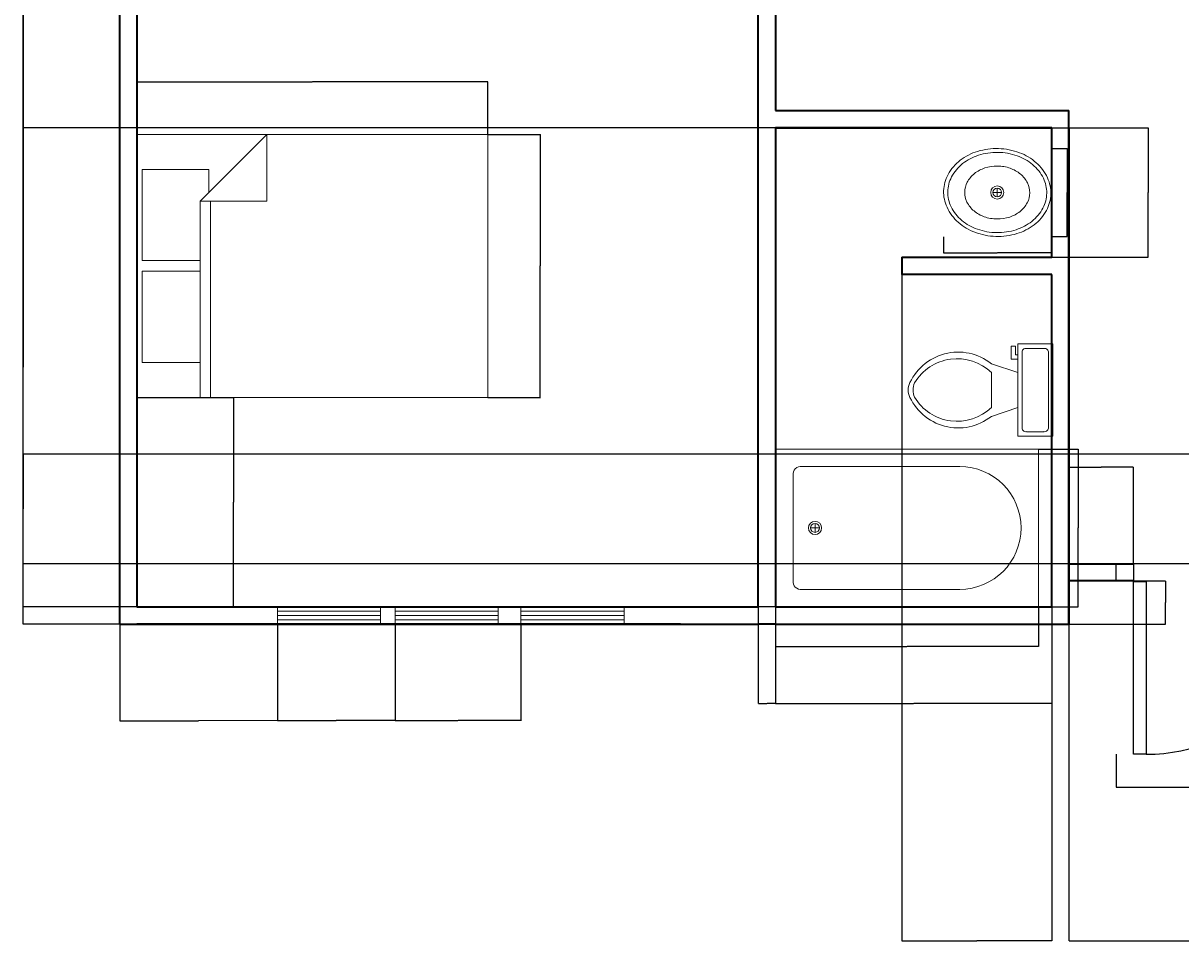
# Model space of a CAD drawing. Units: millimetres. Extents: x 1312 to 12932, y -881 to 10062.
# Tile 1 of 4: x 1312 to 8020, y -881 to 4434. Entities that reach past the tile are written whole.
import ezdxf

# ---------------------------------------------------------------- set-up
doc = ezdxf.new("R2010")
doc.units = ezdxf.units.MM
for name, color, linetype, lineweight in [('A-ANNO-DIMS', 2, 'Continuous', 18), ('A-DOOR', 3, 'Continuous', 25), ('A-FLOR-FIXT', 9, 'Continuous', 18), ('A-FURN', 8, 'Continuous', 18), ('A-GLAZ', 4, 'Continuous', 18), ('A-WALL', 7, 'Continuous', 35)]:
    doc.layers.add(name, color=color, linetype=linetype, lineweight=lineweight)
doc.styles.get("Standard").update_dxf_attribs({"font": 'arial.ttf'})
doc.dimstyles.get("Standard").update_dxf_attribs({"dimtxt": 0.18, "dimasz": 0.18, "dimexe": 0.18, "dimexo": 0.0625, "dimgap": 0.09, "dimtad": 0, "dimtih": 1, "dimtoh": 1, "dimdec": 4, "dimzin": 0, "dimdsep": 46, "dimtxsty": 'Standard', "dimcen": 0.09, "dimadec": 0, "dimazin": 0, "dimtfac": 1, "dimtdec": 4, "dimtofl": 0, "dimtmove": 0, "dimatfit": 3, "dimfxl": 1, "dimtolj": 1, "dimtzin": 0, "dimarcsym": 0})

# ---------------------------------------------------------------- blocks, each defined once
blk = doc.blocks.new('Bed - Queen')
for p, q in [((0, -80.00003), (0, 0)), ((0, 0), (59.99999, 0)), ((59.99999, 0), (59.99999, -80.00003)), ((7.99999, -1.2), (28.79998, -1.2)), ((7.99999, -14.4), (7.99999, -1.2)), ((28.79998, -1.2), (28.79998, -14.4)), ((31.19999, -1.2), (51.99999, -1.2)), ((31.19999, -14.4), (31.19999, -1.2)), ((51.99999, -1.2), (51.99999, -16.4)), ((0, -14.4), (44.8, -14.4)), ((59.99999, -29.6), (44.8, -14.4)), ((44.8, -14.4), (44.8, -29.6)), ((44.8, -16.8), (0, -16.8)), ((51.99999, -16.4), (46.79936, -16.4)), ((44.8, -29.6), (59.99999, -29.6)), ((59.99999, -80.00003), (0, -80.00003))]:
    blk.add_line(p, q)
blk = doc.blocks.new('Toilet - top')
for p, q in [((9.5, -6), (9.5, -2)), ((-10, -8.5), (-8, -8.5)), ((-10, -9.5), (-10, -8.5)), ((-7, -9.5), (-10, -9.5)), ((-8, -8.5), (-8, -8)), ((-7, -8), (-7, -9.5)), ((-4, -8), (-6, -14)), ((4, -8), (6, -14)), ((4, -14), (-4, -14))]:
    blk.add_line(p, q)
blk.add_lwpolyline([(10.5, -8), (10.5, 0), (-10.5, 0), (-10.5, -8)], close=True)
for points in [[(-9.5, -2), (-9.5, -6)], [(8.5, -1), (-8.5, -1)], [(-8.5, -7), (8.5, -7)]]:
    blk.add_lwpolyline(points)
for centre, radius, start, end in [((-8.62, -1.88), 0.884, 81.8699, 188.1301), ((8.62, -1.88), 0.884, 351.8699, 98.1301), ((-8.62, -6.12), 0.884, 171.8699, 278.1301), ((8.62, -6.12), 0.884, 261.8699, 8.1301), ((3.52, -21.58), 12.17, 141.4691, 247.9714), ((4.2, -21.82), 11.33, 136.3677, 238.9468), ((-3.52, -21.58), 12.17, 292.0284, 38.5307), ((-4.2, -21.82), 11.33, 301.053, 43.6321), ((0, -27.88), 4, 245.7318, 294.2682), ((0, -29), 4, 254.8605, 285.1395)]:
    blk.add_arc(centre, radius, start, end)
blk = doc.blocks.new('Bath Tub - 26 x 60 in.')
for p, q in [((8, -18), (10, -18)), ((9, -17), (9, -19))]:
    blk.add_line(p, q)
blk.add_lwpolyline([(0, -36), (0, 0), (60, 0), (60, -36)], close=True)
for points in [[(6, -4), (42, -4)], [(4, -30), (4, -6)], [(42, -32), (6, -32)]]:
    blk.add_lwpolyline(points)
for radius in [1.5, 1]:
    blk.add_circle((9, -18), radius)
for centre, radius, start, end in [((5.75, -5.75), 1.77, 81.8699, 188.1301), ((42, -18), 14, 270, 90), ((5.75, -30.25), 1.77, 171.8699, 278.1301)]:
    blk.add_arc(centre, radius, start, end)
blk = doc.blocks.new('Sink - Oval top')
for p, q in [((-1, 0), (1, 0)), ((0, 1), (0, -1))]:
    blk.add_line(p, q)
for points in [[(-12.23, 0.39, 0.117634), (-11.46, -3.36, 0.104469), (-8.88, -6.8, 0.090016), (-5.08, -9.07, 0.08192), (-0.32, -10.02, 0.08192), (4.49, -9.38, 0.090016), (8.42, -7.36, 0.104469), (11.22, -4.09, 0.117634), (12.23, -0.39, 0.117634), (11.46, 3.36, 0.104469), (8.88, 6.8, 0.090016), (5.08, 9.07, 0.08192), (0.32, 10.02, 0.08192), (-4.49, 9.38, 0.090016), (-8.42, 7.36, 0.104469), (-11.22, 4.09, 0.117634)], [(-11.29, 0.16, 0.118622), (-10.52, -3.25, 0.104678), (-8.07, -6.36, 0.089562), (-4.54, -8.37, 0.081185), (-0.13, -9.15, 0.081185), (4.3, -8.49, 0.089562), (7.89, -6.58, 0.104678), (10.42, -3.55, 0.118622), (11.29, -0.16, 0.118622), (10.52, 3.25, 0.104678), (8.07, 6.36, 0.089562), (4.54, 8.37, 0.081185), (0.13, 9.15, 0.081185), (-4.3, 8.49, 0.089562), (-7.89, 6.58, 0.104678), (-10.42, 3.55, 0.118622)], [(-7.42, 0.08, 0.118283), (-6.91, -2.17, 0.104607), (-5.29, -4.21, 0.089718), (-2.97, -5.53, 0.081436), (-0.07, -6.04, 0.081436), (2.84, -5.59, 0.089718), (5.2, -4.33, 0.104607), (6.86, -2.32, 0.118283), (7.42, -0.08, 0.118283), (6.91, 2.17, 0.104607), (5.29, 4.21, 0.089718), (2.97, 5.53, 0.081436), (0.07, 6.04, 0.081436), (-2.84, 5.59, 0.089718), (-5.2, 4.33, 0.104607), (-6.86, 2.32, 0.118283)]]:
    blk.add_lwpolyline(points, format="xyb", close=True)
for radius in [1.5, 1]:
    blk.add_circle((0, 0), radius)
blk = doc.blocks.new('Window - Wood Frame 36 in. Wide plan')
for p, q in [((0, 6), (0, 0)), ((0, 4.5), (36, 4.5)), ((36, 6), (36, 0)), ((0, 3), (36, 3)), ((0, 1.5), (36, 1.5))]:
    blk.add_line(p, q)
blk = doc.blocks.new('DOOR-SINGLE-1000')
for p, q in [((0, 1003.8), (0, 1103.8)), ((0, 1103.8), (100, 1103.8)), ((100, 1103.8), (100, 1003.8)), ((1174.2, 1000), (1174.2, 1100)), ((1174.2, 1100), (1274.2, 1100)), ((1274.2, 1100), (1274.2, 1000)), ((100, 1003.8), (0, 1003.8)), ((100, 1000), (174.2, 1000)), ((100, 0), (100, 1000)), ((174.2, 1000), (174.2, 0)), ((1274.2, 1000), (1174.2, 1000)), ((174.2, 0), (100, 0))]:
    blk.add_line(p, q)
blk.add_arc((174.2, 1000), 1000, 270, 0)
blk = doc.blocks.new('*D15')
at = {"layer": 'A-ANNO-DIMS', "color": 0, "lineweight": -2, "transparency": 16777216}
for p, q in [((7644.9, 199.3), (7644.9, 8)), ((8919.1, 199.3), (8919.1, 8)), ((7645.1, 8.2), (8280.6, 8.2)), ((8918.9, 8.2), (8283.4, 8.2))]:
    blk.add_line(p, q, dxfattribs=at)
at = {"layer": 'A-ANNO-DIMS', "color": 0, "transparency": 16777216}
for points in [[(7645.1, 8.2), (7645.1, 8.2), (7644.9, 8.2)], [(8918.9, 8.2), (8918.9, 8.2), (8919.1, 8.2)]]:
    blk.add_solid(points, dxfattribs=at)
at = {"layer": 'Defpoints', "color": 0, "transparency": 16777216}
for p in [(7644.9, 199.3), (8919.1, 199.3), (8919.1, 8.2)]:
    blk.add_point(p, dxfattribs=at)
at = {"layer": 'A-ANNO-DIMS', "color": 0, "transparency": 16777216, "insert": (8282, 8.2), "char_height": 0.18, "attachment_point": 5}
blk.add_mtext('\\A1;DOOR UNIT 1274 TYP.', dxfattribs=at)
blk = doc.blocks.new('*D25')
at = {"layer": 'A-ANNO-DIMS', "color": 0, "lineweight": -2, "transparency": 16777216}
for p, q in [((5672, 1053), (5672, 824.3)), ((7196, 1053), (7196, 824.3)), ((5672.2, 824.5), (6433.3, 824.5)), ((7195.8, 824.5), (6434.7, 824.5))]:
    blk.add_line(p, q, dxfattribs=at)
at = {"layer": 'A-ANNO-DIMS', "color": 0, "transparency": 16777216}
for points in [[(5672.2, 824.5), (5672.2, 824.4), (5672, 824.5)], [(7195.8, 824.5), (7195.8, 824.4), (7196, 824.5)]]:
    blk.add_solid(points, dxfattribs=at)
at = {"layer": 'Defpoints', "color": 0, "transparency": 16777216}
for p in [(5672, 1053.1), (7196, 1053.1), (7196, 824.5)]:
    blk.add_point(p, dxfattribs=at)
at = {"layer": 'A-ANNO-DIMS', "color": 0, "transparency": 16777216, "insert": (6434, 824.5), "char_height": 0.18, "attachment_point": 5}
blk.add_mtext('\\A1;BATH 1524', dxfattribs=at)
blk = doc.blocks.new('*D26')
at = {"layer": 'A-ANNO-DIMS', "color": 0, "lineweight": -2, "transparency": 16777216}
for p, q in [((7196.1, 1967.5), (7424.8, 1967.5)), ((7424.6, 1967.3), (7424.6, 1510.4)), ((7424.6, 1053.2), (7424.6, 1510.1)), ((7196.1, 1053.1), (7424.8, 1053.1))]:
    blk.add_line(p, q, dxfattribs=at)
at = {"layer": 'A-ANNO-DIMS', "color": 0, "transparency": 16777216}
for points in [[(7424.6, 1967.3), (7424.6, 1967.3), (7424.6, 1967.5)], [(7424.6, 1053.2), (7424.6, 1053.2), (7424.6, 1053.1)]]:
    blk.add_solid(points, dxfattribs=at)
at = {"layer": 'Defpoints', "color": 0, "transparency": 16777216}
for p in [(7196, 1967.5), (7424.6, 1967.5), (7196, 1053.1)]:
    blk.add_point(p, dxfattribs=at)
at = {"layer": 'A-ANNO-DIMS', "color": 0, "transparency": 16777216, "insert": (7424.6, 1510.3), "char_height": 0.18, "attachment_point": 5}
blk.add_mtext('\\A1;914', dxfattribs=at)
blk = doc.blocks.new('*D27')
at = {"layer": 'A-ANNO-DIMS', "color": 0, "lineweight": -2, "transparency": 16777216}
for p, q in [((1972, 3790.1), (1972, 4095)), ((1972.2, 4094.9), (2986.5, 4094.9)), ((4003.8, 4094.9), (2989.4, 4094.9)), ((4004, 3790.1), (4004, 4095))]:
    blk.add_line(p, q, dxfattribs=at)
at = {"layer": 'A-ANNO-DIMS', "color": 0, "transparency": 16777216}
for points in [[(1972.2, 4094.9), (1972.2, 4094.8), (1972, 4094.9)], [(4003.8, 4094.9), (4003.8, 4094.8), (4004, 4094.9)]]:
    blk.add_solid(points, dxfattribs=at)
at = {"layer": 'Defpoints', "color": 0, "transparency": 16777216}
for p in [(1972, 4094.9), (1972, 3790.1), (4004, 3790.1)]:
    blk.add_point(p, dxfattribs=at)
at = {"layer": 'A-ANNO-DIMS', "color": 0, "transparency": 16777216, "insert": (2988, 4094.9), "char_height": 0.18, "attachment_point": 5}
blk.add_mtext('\\A1;QUEEN BED 2032 TYP.', dxfattribs=at)
blk = doc.blocks.new('*D28')
at = {"layer": 'A-ANNO-DIMS', "color": 0, "lineweight": -2, "transparency": 16777216}
for p, q in [((4004.1, 3790.1), (4309, 3790.1)), ((4308.8, 3789.9), (4308.8, 3028.2)), ((4308.8, 2266.2), (4308.8, 3027.9)), ((4004.1, 2266.1), (4309, 2266.1))]:
    blk.add_line(p, q, dxfattribs=at)
at = {"layer": 'A-ANNO-DIMS', "color": 0, "transparency": 16777216}
for points in [[(4308.8, 3789.9), (4308.8, 3789.9), (4308.8, 3790.1)], [(4308.8, 2266.2), (4308.8, 2266.2), (4308.8, 2266.1)]]:
    blk.add_solid(points, dxfattribs=at)
at = {"layer": 'Defpoints', "color": 0, "transparency": 16777216}
for p in [(4004, 3790.1), (4308.8, 3790.1), (4004, 2266.1)]:
    blk.add_point(p, dxfattribs=at)
at = {"layer": 'A-ANNO-DIMS', "color": 0, "transparency": 16777216, "insert": (4308.8, 3028.1), "char_height": 0.18, "attachment_point": 5}
blk.add_mtext('\\A1;1524 TYP.', dxfattribs=at)
blk = doc.blocks.new('*D31')
at = {"layer": 'A-ANNO-DIMS', "color": 0, "lineweight": -2, "transparency": 16777216}
for p, q in [((6644.5, 3197.5), (6644.5, 3103.9)), ((7268.1, 3197.5), (7268.1, 3103.9)), ((6644.7, 3104.1), (6955.6, 3104.1)), ((7267.9, 3104.1), (6957, 3104.1))]:
    blk.add_line(p, q, dxfattribs=at)
at = {"layer": 'A-ANNO-DIMS', "color": 0, "transparency": 16777216}
for points in [[(6644.7, 3104.1), (6644.7, 3104), (6644.5, 3104.1)], [(7267.9, 3104.1), (7267.9, 3104), (7268.1, 3104.1)]]:
    blk.add_solid(points, dxfattribs=at)
at = {"layer": 'Defpoints', "color": 0, "transparency": 16777216}
for p in [(6644.5, 3197.6), (7268.1, 3197.6), (7268.1, 3104.1)]:
    blk.add_point(p, dxfattribs=at)
at = {"layer": 'A-ANNO-DIMS', "color": 0, "transparency": 16777216, "insert": (6956.3, 3104.1), "char_height": 0.18, "attachment_point": 5}
blk.add_mtext('\\A1;BASIN 624', dxfattribs=at)
blk = doc.blocks.new('*D32')
at = {"layer": 'A-ANNO-DIMS', "color": 0, "lineweight": -2, "transparency": 16777216}
for p, q in [((7268.2, 3709.1), (7361.8, 3709.1)), ((7361.6, 3708.9), (7361.6, 3453.5)), ((7361.6, 3197.8), (7361.6, 3453.2)), ((7268.2, 3197.6), (7361.8, 3197.6))]:
    blk.add_line(p, q, dxfattribs=at)
at = {"layer": 'A-ANNO-DIMS', "color": 0, "transparency": 16777216}
for points in [[(7361.6, 3708.9), (7361.7, 3708.9), (7361.6, 3709.1)], [(7361.6, 3197.8), (7361.7, 3197.8), (7361.6, 3197.6)]]:
    blk.add_solid(points, dxfattribs=at)
at = {"layer": 'Defpoints', "color": 0, "transparency": 16777216}
for p in [(7268.1, 3709.1), (7361.6, 3709.1), (7268.1, 3197.6)]:
    blk.add_point(p, dxfattribs=at)
at = {"layer": 'A-ANNO-DIMS', "color": 0, "transparency": 16777216, "insert": (7361.6, 3453.3), "char_height": 0.18, "attachment_point": 5}
blk.add_mtext('\\A1;511', dxfattribs=at)
blk = doc.blocks.new('*D42')
at = {"layer": 'A-ANNO-DIMS', "color": 0, "lineweight": -2, "transparency": 16777216}
for p, q in [((1876.6, 9503.1), (1312.6, 9503.1)), ((1312.7, 9502.9), (1312.7, 5228.2)), ((1312.7, 953.2), (1312.7, 5227.9)), ((1871.9, 953.1), (1312.6, 953.1))]:
    blk.add_line(p, q, dxfattribs=at)
at = {"layer": 'A-ANNO-DIMS', "color": 0, "transparency": 16777216}
for points in [[(1312.7, 9502.9), (1312.8, 9502.9), (1312.7, 9503.1)], [(1312.7, 953.2), (1312.8, 953.2), (1312.7, 953.1)]]:
    blk.add_solid(points, dxfattribs=at)
at = {"layer": 'Defpoints', "color": 0, "transparency": 16777216}
for p in [(1312.7, 9503.1), (1876.6, 9503.1), (1872, 953.1)]:
    blk.add_point(p, dxfattribs=at)
at = {"layer": 'A-ANNO-DIMS', "color": 0, "transparency": 16777216, "insert": (1312.7, 5228.1), "char_height": 0.18, "attachment_point": 5}
blk.add_mtext('\\A1;8550', dxfattribs=at)
blk = doc.blocks.new('*D47')
at = {"layer": 'A-ANNO-DIMS', "color": 0, "lineweight": -2, "transparency": 16777216}
for p, q in [((1971.9, 5103.1), (1312.6, 5103.1)), ((1312.7, 5102.9), (1312.7, 3078.2)), ((1312.7, 1053.2), (1312.7, 3077.9)), ((1971.9, 1053.1), (1312.6, 1053.1))]:
    blk.add_line(p, q, dxfattribs=at)
at = {"layer": 'A-ANNO-DIMS', "color": 0, "transparency": 16777216}
for points in [[(1312.7, 5102.9), (1312.8, 5102.9), (1312.7, 5103.1)], [(1312.7, 1053.2), (1312.8, 1053.2), (1312.7, 1053.1)]]:
    blk.add_solid(points, dxfattribs=at)
at = {"layer": 'Defpoints', "color": 0, "transparency": 16777216}
for p in [(1312.7, 5103.1), (1972, 5103.1), (1972, 1053.1)]:
    blk.add_point(p, dxfattribs=at)
at = {"layer": 'A-ANNO-DIMS', "color": 0, "transparency": 16777216, "insert": (1312.7, 3078.1), "char_height": 0.18, "attachment_point": 5}
blk.add_mtext('\\A1;4050', dxfattribs=at)
blk = doc.blocks.new('*D51')
at = {"layer": 'A-ANNO-DIMS', "color": 0, "lineweight": -2, "transparency": 16777216}
for p, q in [((5672, 1053), (5672, 493.6)), ((7272, 1053), (7272, 493.6)), ((5672.2, 493.8), (6471.6, 493.8)), ((7271.8, 493.8), (6472.3, 493.8))]:
    blk.add_line(p, q, dxfattribs=at)
at = {"layer": 'A-ANNO-DIMS', "color": 0, "transparency": 16777216}
for points in [[(5672.2, 493.8), (5672.2, 493.8), (5672, 493.8)], [(7271.8, 493.8), (7271.8, 493.8), (7272, 493.8)]]:
    blk.add_solid(points, dxfattribs=at)
at = {"layer": 'Defpoints', "color": 0, "transparency": 16777216}
for p in [(5672, 1053.1), (7272, 1053.1), (5672, 493.8)]:
    blk.add_point(p, dxfattribs=at)
at = {"layer": 'A-ANNO-DIMS', "color": 0, "transparency": 16777216, "insert": (6472, 493.8), "char_height": 0.18, "attachment_point": 5}
blk.add_mtext('\\A1;1600', dxfattribs=at)
blk = doc.blocks.new('*D52')
at = {"layer": 'A-ANNO-DIMS', "color": 0, "lineweight": -2, "transparency": 16777216}
for p, q in [((5572, 1053), (5572, 493.6)), ((5672, 1053), (5672, 493.6)), ((5572.2, 493.8), (5621.7, 493.8)), ((5671.8, 493.8), (5622.3, 493.8))]:
    blk.add_line(p, q, dxfattribs=at)
at = {"layer": 'A-ANNO-DIMS', "color": 0, "transparency": 16777216}
for points in [[(5572.2, 493.8), (5572.2, 493.8), (5572, 493.8)], [(5671.8, 493.8), (5671.8, 493.8), (5672, 493.8)]]:
    blk.add_solid(points, dxfattribs=at)
at = {"layer": 'Defpoints', "color": 0, "transparency": 16777216}
for p in [(5572, 1053.1), (5672, 1053.1), (5572, 493.8)]:
    blk.add_point(p, dxfattribs=at)
at = {"layer": 'A-ANNO-DIMS', "color": 0, "transparency": 16777216, "insert": (5622, 493.8), "char_height": 0.18, "attachment_point": 5}
blk.add_mtext('\\A1;100', dxfattribs=at)
blk = doc.blocks.new('*D53')
at = {"layer": 'A-ANNO-DIMS', "color": 0, "lineweight": -2, "transparency": 16777216}
for p, q in [((5671.9, 3828.5), (1312.6, 3828.5)), ((1312.7, 3828.3), (1312.7, 2441)), ((1312.7, 1053.2), (1312.7, 2440.6)), ((5671.9, 1053.1), (1312.6, 1053.1))]:
    blk.add_line(p, q, dxfattribs=at)
at = {"layer": 'A-ANNO-DIMS', "color": 0, "transparency": 16777216}
for points in [[(1312.7, 3828.3), (1312.8, 3828.3), (1312.7, 3828.5)], [(1312.7, 1053.2), (1312.8, 1053.2), (1312.7, 1053.1)]]:
    blk.add_solid(points, dxfattribs=at)
at = {"layer": 'Defpoints', "color": 0, "transparency": 16777216}
for p in [(1312.7, 3828.5), (5672, 3828.5), (5672, 1053.1)]:
    blk.add_point(p, dxfattribs=at)
at = {"layer": 'A-ANNO-DIMS', "color": 0, "transparency": 16777216, "insert": (1312.7, 2440.8), "char_height": 0.18, "attachment_point": 5}
blk.add_mtext('\\A1;2775.4', dxfattribs=at)
blk = doc.blocks.new('*D59')
at = {"layer": 'A-ANNO-DIMS', "color": 0, "lineweight": -2, "transparency": 16777216}
for p, q in [((7372, 1203), (7372, -881.3)), ((12372, 1203), (12372, -881.3)), ((7372.2, -881.1), (9871.6, -881.1)), ((12371.8, -881.1), (9872.4, -881.1))]:
    blk.add_line(p, q, dxfattribs=at)
at = {"layer": 'A-ANNO-DIMS', "color": 0, "transparency": 16777216}
for points in [[(7372.2, -881), (7372.2, -881.1), (7372, -881.1)], [(12371.8, -881), (12371.8, -881.1), (12372, -881.1)]]:
    blk.add_solid(points, dxfattribs=at)
at = {"layer": 'Defpoints', "color": 0, "transparency": 16777216}
for p in [(7372, 1203.1), (12372, 1203.1), (12372, -881.1)]:
    blk.add_point(p, dxfattribs=at)
at = {"layer": 'A-ANNO-DIMS', "color": 0, "transparency": 16777216, "insert": (9872, -881.1), "char_height": 0.18, "attachment_point": 5}
blk.add_mtext('\\A1;5000', dxfattribs=at)
blk = doc.blocks.new('*D60')
at = {"layer": 'A-ANNO-DIMS', "color": 0, "lineweight": -2, "transparency": 16777216}
for p, q in [((7372, 1303.2), (7372, 1862.5)), ((7372.2, 1862.3), (7558.1, 1862.3)), ((7744.7, 1862.3), (7558.8, 1862.3)), ((7744.9, 1303.2), (7744.9, 1862.5))]:
    blk.add_line(p, q, dxfattribs=at)
at = {"layer": 'A-ANNO-DIMS', "color": 0, "transparency": 16777216}
for points in [[(7372.2, 1862.4), (7372.2, 1862.3), (7372, 1862.3)], [(7744.7, 1862.4), (7744.7, 1862.3), (7744.9, 1862.3)]]:
    blk.add_solid(points, dxfattribs=at)
at = {"layer": 'Defpoints', "color": 0, "transparency": 16777216}
for p in [(7744.9, 1862.3), (7372, 1303.1), (7744.9, 1303.1)]:
    blk.add_point(p, dxfattribs=at)
at = {"layer": 'A-ANNO-DIMS', "color": 0, "transparency": 16777216, "insert": (7558.4, 1862.3), "char_height": 0.18, "attachment_point": 5}
blk.add_mtext('\\A1;372.9', dxfattribs=at)
blk = doc.blocks.new('*D61')
at = {"layer": 'A-ANNO-DIMS', "color": 0, "lineweight": -2, "transparency": 16777216}
for p, q in [((7372.1, 1203.1), (7931.4, 1203.1)), ((7931.2, 1202.9), (7931.2, 1078.3)), ((7931.2, 953.2), (7931.2, 1077.9)), ((7372.1, 953.1), (7931.4, 953.1))]:
    blk.add_line(p, q, dxfattribs=at)
at = {"layer": 'A-ANNO-DIMS', "color": 0, "transparency": 16777216}
for points in [[(7931.2, 1202.9), (7931.3, 1202.9), (7931.2, 1203.1)], [(7931.2, 953.2), (7931.3, 953.2), (7931.2, 953.1)]]:
    blk.add_solid(points, dxfattribs=at)
at = {"layer": 'Defpoints', "color": 0, "transparency": 16777216}
for p in [(7372, 1203.1), (7372, 953.1), (7931.2, 953.1)]:
    blk.add_point(p, dxfattribs=at)
at = {"layer": 'A-ANNO-DIMS', "color": 0, "transparency": 16777216, "insert": (7931.2, 1078.1), "char_height": 0.18, "attachment_point": 5}
blk.add_mtext('\\A1;250.03', dxfattribs=at)
blk = doc.blocks.new('*D69')
at = {"layer": 'A-ANNO-DIMS', "color": 0, "lineweight": -2, "transparency": 16777216}
for p, q in [((1872, 953), (1872.2, 393.6)), ((2785.1, 953.3), (2785.3, 394)), ((1872.4, 393.8), (2328.4, 394)), ((2785.1, 394.1), (2329.1, 394))]:
    blk.add_line(p, q, dxfattribs=at)
at = {"layer": 'A-ANNO-DIMS', "color": 0, "transparency": 16777216}
for points in [[(1872.4, 393.8), (1872.4, 393.8), (1872.2, 393.8)], [(2785.1, 394.2), (2785.1, 394.1), (2785.3, 394.1)]]:
    blk.add_solid(points, dxfattribs=at)
at = {"layer": 'Defpoints', "color": 0, "transparency": 16777216}
for p in [(1872, 953.1), (2785.1, 953.4), (1872.2, 393.8)]:
    blk.add_point(p, dxfattribs=at)
at = {"layer": 'A-ANNO-DIMS', "color": 0, "transparency": 16777216, "insert": (2328.8, 394), "char_height": 0.18, "attachment_point": 5}
blk.add_mtext('\\A1;913.1', dxfattribs=at)
blk = doc.blocks.new('*D70')
at = {"layer": 'A-ANNO-DIMS', "color": 0, "lineweight": -2, "transparency": 16777216}
for p, q in [((2785.1, 953.3), (2785.1, 394)), ((3467.5, 953.3), (3467.5, 394)), ((2785.3, 394.1), (3125.9, 394.1)), ((3467.3, 394.1), (3126.7, 394.1))]:
    blk.add_line(p, q, dxfattribs=at)
at = {"layer": 'A-ANNO-DIMS', "color": 0, "transparency": 16777216}
for points in [[(2785.3, 394.2), (2785.3, 394.1), (2785.1, 394.1)], [(3467.3, 394.2), (3467.3, 394.1), (3467.5, 394.1)]]:
    blk.add_solid(points, dxfattribs=at)
at = {"layer": 'Defpoints', "color": 0, "transparency": 16777216}
for p in [(2785.1, 953.4), (3467.5, 953.4), (2785.1, 394.1)]:
    blk.add_point(p, dxfattribs=at)
at = {"layer": 'A-ANNO-DIMS', "color": 0, "transparency": 16777216, "insert": (3126.3, 394.1), "char_height": 0.18, "attachment_point": 5}
blk.add_mtext('\\A1;682.3', dxfattribs=at)
blk = doc.blocks.new('*D71')
at = {"layer": 'A-ANNO-DIMS', "color": 0, "lineweight": -2, "transparency": 16777216}
for p, q in [((3467.5, 953.3), (3467.5, 394)), ((4196.3, 953.3), (4196.3, 394)), ((3467.6, 394.1), (3831.5, 394.1)), ((4196.1, 394.1), (3832.3, 394.1))]:
    blk.add_line(p, q, dxfattribs=at)
at = {"layer": 'A-ANNO-DIMS', "color": 0, "transparency": 16777216}
for points in [[(3467.6, 394.2), (3467.6, 394.1), (3467.5, 394.1)], [(4196.1, 394.2), (4196.1, 394.1), (4196.3, 394.1)]]:
    blk.add_solid(points, dxfattribs=at)
at = {"layer": 'Defpoints', "color": 0, "transparency": 16777216}
for p in [(3467.5, 953.4), (4196.3, 953.4), (3467.5, 394.1)]:
    blk.add_point(p, dxfattribs=at)
at = {"layer": 'A-ANNO-DIMS', "color": 0, "transparency": 16777216, "insert": (3831.9, 394.1), "char_height": 0.18, "attachment_point": 5}
blk.add_mtext('\\A1;728.9', dxfattribs=at)
blk = doc.blocks.new('*D83')
at = {"layer": 'A-ANNO-DIMS', "color": 0, "lineweight": -2, "transparency": 16777216}
for p, q in [((1972.1, 2266.1), (2531.4, 2266.1)), ((2531.2, 2265.9), (2531.2, 1659.7)), ((2531.2, 1053.2), (2531.2, 1659.4)), ((1972.1, 1053.1), (2531.4, 1053.1))]:
    blk.add_line(p, q, dxfattribs=at)
at = {"layer": 'A-ANNO-DIMS', "color": 0, "transparency": 16777216}
for points in [[(2531.2, 2265.9), (2531.3, 2265.9), (2531.2, 2266.1)], [(2531.2, 1053.2), (2531.3, 1053.2), (2531.2, 1053.1)]]:
    blk.add_solid(points, dxfattribs=at)
at = {"layer": 'Defpoints', "color": 0, "transparency": 16777216}
for p in [(1972, 2266.1), (1972, 1053.1), (2531.2, 1053.1)]:
    blk.add_point(p, dxfattribs=at)
at = {"layer": 'A-ANNO-DIMS', "color": 0, "transparency": 16777216, "insert": (2531.2, 1659.6), "char_height": 0.18, "attachment_point": 5}
blk.add_mtext('\\A1;1213', dxfattribs=at)
blk = doc.blocks.new('*D87')
at = {"layer": 'A-ANNO-DIMS', "color": 0, "lineweight": -2, "transparency": 16777216}
for p, q in [((6403.3, 2978.2), (6403.3, -881.3)), ((7272, 2978.2), (7272, -881.3)), ((6403.5, -881.1), (6837.3, -881.1)), ((7271.8, -881.1), (6838.1, -881.1))]:
    blk.add_line(p, q, dxfattribs=at)
at = {"layer": 'A-ANNO-DIMS', "color": 0, "transparency": 16777216}
for points in [[(6403.5, -881), (6403.5, -881.1), (6403.3, -881.1)], [(7271.8, -881), (7271.8, -881.1), (7272, -881.1)]]:
    blk.add_solid(points, dxfattribs=at)
at = {"layer": 'Defpoints', "color": 0, "transparency": 16777216}
for p in [(6403.3, 2978.2), (7272, 2978.2), (6403.3, -881.1)]:
    blk.add_point(p, dxfattribs=at)
at = {"layer": 'A-ANNO-DIMS', "color": 0, "transparency": 16777216, "insert": (6837.7, -881.1), "char_height": 0.18, "attachment_point": 5}
blk.add_mtext('\\A1;868.7', dxfattribs=at)
blk = doc.blocks.new('*D88')
at = {"layer": 'A-ANNO-DIMS', "color": 0, "lineweight": -2, "transparency": 16777216}
for p, q in [((7272.1, 3828.5), (7831.4, 3828.5)), ((7831.2, 3828.3), (7831.2, 3453.5)), ((7831.2, 3078.4), (7831.2, 3453.2)), ((7272.1, 3078.2), (7831.4, 3078.2))]:
    blk.add_line(p, q, dxfattribs=at)
at = {"layer": 'A-ANNO-DIMS', "color": 0, "transparency": 16777216}
for points in [[(7831.2, 3828.3), (7831.3, 3828.3), (7831.2, 3828.5)], [(7831.2, 3078.4), (7831.3, 3078.4), (7831.2, 3078.2)]]:
    blk.add_solid(points, dxfattribs=at)
at = {"layer": 'Defpoints', "color": 0, "transparency": 16777216}
for p in [(7272, 3828.5), (7272, 3078.2), (7831.2, 3078.2)]:
    blk.add_point(p, dxfattribs=at)
at = {"layer": 'A-ANNO-DIMS', "color": 0, "transparency": 16777216, "insert": (7831.2, 3453.4), "char_height": 0.18, "attachment_point": 5}
blk.add_mtext('\\A1;750.3', dxfattribs=at)
blk = doc.blocks.new('*D96')
at = {"layer": 'A-ANNO-DIMS', "color": 0, "lineweight": -2, "transparency": 16777216}
for p, q in [((11773.9, 1938.6), (1312.6, 1938.6)), ((1312.7, 1938.4), (1312.7, 1621)), ((1312.7, 1303.3), (1312.7, 1620.7)), ((12271.9, 1303.1), (1312.6, 1303.1))]:
    blk.add_line(p, q, dxfattribs=at)
at = {"layer": 'A-ANNO-DIMS', "color": 0, "transparency": 16777216}
for points in [[(1312.7, 1938.4), (1312.8, 1938.4), (1312.7, 1938.6)], [(1312.7, 1303.3), (1312.8, 1303.3), (1312.7, 1303.1)]]:
    blk.add_solid(points, dxfattribs=at)
at = {"layer": 'Defpoints', "color": 0, "transparency": 16777216}
for p in [(11774, 1938.6), (1312.7, 1303.1), (12272, 1303.1)]:
    blk.add_point(p, dxfattribs=at)
at = {"layer": 'A-ANNO-DIMS', "color": 0, "transparency": 16777216, "insert": (1312.7, 1620.8), "char_height": 0.18, "attachment_point": 5}
blk.add_mtext('\\A1;635.5', dxfattribs=at)
blk = doc.blocks.new('*D98')
at = {"layer": 'A-ANNO-DIMS', "color": 0, "lineweight": -2, "transparency": 16777216}
for p, q in [((7819, 1199.3), (7819.2, 1199.3)), ((7819.1, 1199.2), (7819.1, 1199.4)), ((8950.5, 67.9), (8526.3, 492.1)), ((8950.6, 67.9), (8950.5, 67.9))]:
    blk.add_line(p, q, dxfattribs=at)
at = {"layer": 'A-ANNO-DIMS', "color": 0, "transparency": 16777216}
blk.add_solid([(8526.4, 492.1), (8526.3, 492.1), (8526.2, 492.2)], dxfattribs=at)
at = {"layer": 'Defpoints', "color": 0, "transparency": 16777216}
for p in [(7819.1, 1199.3), (8526.2, 492.2)]:
    blk.add_point(p, dxfattribs=at)
at = {"layer": 'A-ANNO-DIMS', "color": 0, "transparency": 16777216, "insert": (8951.3, 67.9), "char_height": 0.18, "attachment_point": 5}
blk.add_mtext('\\A1;6X R1000', dxfattribs=at)

msp = doc.modelspace()

# ---------------------------------------------------------------- linework, layer by layer
at = {"layer": 'A-WALL'}
for p, q in [((1871.992, 953.061), (1871.992, 9403.061)), ((5571.992, 1053.061), (5571.992, 9403.061)), ((5671.992, 6253.061), (5671.992, 3928.492)), ((1971.992, 5103.061), (1971.992, 1053.061)), ((1971.992, 5103.061), (1971.992, 1053.061)), ((5571.992, 1053.061), (5571.992, 5103.061)), ((5671.992, 3928.492), (7371.992, 3928.492)), ((7371.992, 3828.492), (7371.992, 3928.492)), ((5671.992, 3828.492), (7271.992, 3828.492)), ((7271.992, 3828.492), (5671.992, 3828.492)), ((7271.992, 3828.492), (5671.992, 3828.492)), ((5671.992, 3828.492), (5671.992, 1053.061)), ((7271.992, 3078.232), (7271.992, 3828.492)), ((7371.992, 1203.088), (7371.992, 3828.492)), ((7371.992, 3828.492), (7371.992, 953.061)), ((6403.33, 3078.232), (7271.992, 3078.232)), ((6403.33, 3078.232), (6403.33, 2978.232)), ((7271.992, 2978.232), (6403.33, 2978.232)), ((7271.992, 1053.061), (7271.992, 2978.232)), ((7371.992, 1303.088), (7744.896, 1303.088)), ((7371.992, 953.061), (7371.992, 1203.088)), ((7744.896, 1203.088), (7371.992, 1203.088)), ((7744.896, 1203.088), (7371.992, 1203.088)), ((1971.992, 1053.061), (5121.992, 1053.061)), ((5121.992, 1053.061), (5571.992, 1053.061)), ((5671.992, 1053.061), (7271.992, 1053.061)), ((1871.992, 953.061), (1971.992, 953.061)), ((1971.992, 953.061), (5571.992, 953.061)), ((5121.992, 953.061), (1971.992, 953.061)), ((5671.992, 953.061), (5571.992, 953.061)), ((5671.992, 953.061), (7371.992, 953.061))]:
    msp.add_line(p, q, dxfattribs=at)

# ---------------------------------------------------------------- block references
at = {"layer": 'A-DOOR'}
msp.add_blockref('DOOR-SINGLE-1000', (7644.896, 199.32), dxfattribs=at)
at = {"layer": 'A-FLOR-FIXT', "xscale": 25.4, "yscale": 25.4, "zscale": 25.4}
for name, p in [('Sink - Oval top', (6956.305, 3453.347)), ('Bath Tub - 26 x 60 in.', (5671.992, 1967.461))]:
    msp.add_blockref(name, p, dxfattribs=at)
at = {"layer": 'A-FLOR-FIXT', "xscale": 25.4, "yscale": 25.4, "zscale": 25.4, "rotation": 270}
msp.add_blockref('Toilet - top', (7277.994, 2309.224), dxfattribs=at)
at = {"layer": 'A-FURN', "xscale": 25.4, "yscale": 25.4, "zscale": 25.4, "rotation": 90}
msp.add_blockref('Bed - Queen', (1971.992, 2266.061), dxfattribs=at)
at = {"layer": 'A-GLAZ', "xscale": 16.61312414671267, "yscale": 16.61312414671267, "zscale": 16.61312414671267}
for p in [(2785.115, 953.382), (3467.458, 953.382), (4196.326, 953.382)]:
    msp.add_blockref('Window - Wood Frame 36 in. Wide plan', p, dxfattribs=at)

# ---------------------------------------------------------------- dimensions: what is measured, and where the dimension line sits
at = {"layer": 'A-ANNO-DIMS'}
for base, p1, p2, angle, override, picture, middle in [((1312.742, 9503.061), (1871.992, 953.061), (1876.635, 9503.061), 90, {"dimdec": 0, "dimlfac": 1, "dimrnd": 0, "dimzin": 0, "dimdsep": 46, "dimlunit": 2}, '*D42', (1312.742, 5228.061)), ((1312.742, 5103.061), (1971.992, 1053.061), (1971.992, 5103.061), 90, {"dimdec": 0, "dimlfac": 1, "dimrnd": 0, "dimzin": 0, "dimdsep": 46, "dimlunit": 2}, '*D47', (1312.742, 3078.061)), ((1312.742, 3828.492), (5671.992, 1053.061), (5671.992, 3828.492), 90, {"dimdec": 1, "dimlfac": 1, "dimrnd": 0, "dimzin": 0, "dimdsep": 46, "dimlunit": 2}, '*D53', (1312.742, 2440.776)), ((7831.242, 3078.232), (7271.992, 3828.492), (7271.992, 3078.232), 270, {"dimdec": 1, "dimlfac": 1, "dimrnd": 0, "dimzin": 0, "dimdsep": 46, "dimlunit": 2}, '*D88', (7831.242, 3453.362)), ((7361.641, 3709.082), (7268.102, 3197.612), (7268.102, 3709.082), 90, {"dimdec": 0, "dimlfac": 1, "dimrnd": 0, "dimzin": 0, "dimdsep": 46, "dimlunit": 2}, '*D32', (7361.641, 3453.347)), ((2531.242, 1053.061), (1971.992, 2266.061), (1971.992, 1053.061), 270, {"dimdec": 0, "dimlfac": 1, "dimrnd": 0, "dimzin": 0, "dimdsep": 46, "dimlunit": 2}, '*D83', (2531.242, 1659.561)), ((7424.592, 1967.461), (7195.992, 1053.061), (7195.992, 1967.461), 90, {"dimdec": 0, "dimlfac": 1, "dimrnd": 0, "dimzin": 0, "dimdsep": 46, "dimlunit": 2}, '*D26', (7424.592, 1510.261)), ((1312.742, 1303.088), (11774.012, 1938.594), (12271.992, 1303.088), 90, {"dimdec": 1, "dimlfac": 1, "dimrnd": 0, "dimzin": 0, "dimdsep": 46, "dimlunit": 2}, '*D96', (1312.742, 1620.841)), ((7931.242, 953.061), (7371.992, 1203.088), (7371.992, 953.061), 270, {"dimdec": 2, "dimlfac": 1, "dimrnd": 0, "dimzin": 0, "dimdsep": 46, "dimlunit": 2}, '*D61', (7931.242, 1078.075)), ((5571.992, 493.811), (5671.992, 1053.061), (5571.992, 1053.061), 180, {"dimdec": 0, "dimlfac": 1, "dimrnd": 0, "dimzin": 0, "dimdsep": 46, "dimlunit": 2}, '*D52', (5621.992, 493.811)), ((5671.992, 493.811), (7271.992, 1053.061), (5671.992, 1053.061), 180, {"dimdec": 0, "dimlfac": 1, "dimrnd": 0, "dimzin": 0, "dimdsep": 46, "dimlunit": 2}, '*D51', (6471.992, 493.811)), ((1872.189, 393.811), (2785.115, 953.382), (1871.992, 953.061), 180.0201578, {"dimdec": 1, "dimlfac": 1, "dimrnd": 0, "dimzin": 0, "dimdsep": 46, "dimlunit": 2}, '*D69', (2328.75, 393.972)), ((2785.115, 394.132), (3467.458, 953.382), (2785.115, 953.382), 180, {"dimdec": 1, "dimlfac": 1, "dimrnd": 0, "dimzin": 0, "dimdsep": 46, "dimlunit": 2}, '*D70', (3126.287, 394.132)), ((3467.458, 394.132), (4196.326, 953.382), (3467.458, 953.382), 180, {"dimdec": 1, "dimlfac": 1, "dimrnd": 0, "dimzin": 0, "dimdsep": 46, "dimlunit": 2}, '*D71', (3831.892, 394.132))]:
    dim = msp.add_linear_dim(base=base, p1=p1, p2=p2, angle=angle, dimstyle='Standard', override=override, dxfattribs=at)
    dim.commit()
    dim.dimension.update_dxf_attribs({"geometry": picture, "text_midpoint": middle})
for base, p1, p2, angle, text, picture, middle in [((1971.992, 4094.861), (4003.993, 3790.061), (1971.992, 3790.061), 180, 'QUEEN BED <> TYP.', '*D27', (2987.993, 4094.861)), ((4308.793, 3790.061), (4003.993, 2266.061), (4003.993, 3790.061), 90, '<> TYP.', '*D28', (4308.793, 3028.061))]:
    dim = msp.add_linear_dim(base=base, p1=p1, p2=p2, angle=angle, text=text, dimstyle='Standard', override={"dimdec": 0, "dimlfac": 1, "dimrnd": 0, "dimzin": 0, "dimdsep": 46, "dimlunit": 2}, dxfattribs=at)
    dim.commit()
    dim.dimension.update_dxf_attribs({"geometry": picture, "text_midpoint": middle})
for base, p1, p2, text, picture, middle in [((7268.102, 3104.073), (6644.509, 3197.612), (7268.102, 3197.612), 'BASIN <>', '*D31', (6956.305, 3104.073)), ((7195.992, 824.461), (5671.992, 1053.061), (7195.992, 1053.061), 'BATH <>', '*D25', (6433.992, 824.461)), ((8919.096, 8.19), (7644.896, 199.32), (8919.096, 199.32), 'DOOR UNIT <> TYP.', '*D15', (8281.996, 8.19))]:
    dim = msp.add_linear_dim(base=base, p1=p1, p2=p2, text=text, dimstyle='Standard', override={"dimdec": 0, "dimlfac": 1, "dimrnd": 0, "dimzin": 0, "dimdsep": 46, "dimlunit": 2}, dxfattribs=at)
    dim.commit()
    dim.dimension.update_dxf_attribs({"geometry": picture, "text_midpoint": middle})
for base, p1, p2, override, picture, middle in [((6403.33, -881.079), (7271.992, 2978.232), (6403.33, 2978.232), {"dimdec": 1, "dimlfac": 1, "dimrnd": 0, "dimzin": 0, "dimdsep": 46, "dimlunit": 2}, '*D87', (6837.661, -881.079)), ((7744.896, 1862.338), (7371.992, 1303.088), (7744.896, 1303.088), {"dimdec": 1, "dimlfac": 1, "dimrnd": 0, "dimzin": 0, "dimdsep": 46, "dimlunit": 2}, '*D60', (7558.444, 1862.338)), ((12371.992, -881.079), (7371.992, 1203.088), (12371.992, 1203.088), {"dimdec": 0, "dimlfac": 1, "dimrnd": 0, "dimzin": 0, "dimdsep": 46, "dimlunit": 2}, '*D59', (9871.992, -881.079))]:
    dim = msp.add_linear_dim(base=base, p1=p1, p2=p2, dimstyle='Standard', override=override, dxfattribs=at)
    dim.commit()
    dim.dimension.update_dxf_attribs({"geometry": picture, "text_midpoint": middle})
dim = msp.add_radius_dim(center=(7819.096, 1199.32), mpoint=(8526.203, 492.213), text='6X <>', dimstyle='Standard', override={"dimdec": 0, "dimlfac": 1, "dimrnd": 0, "dimzin": 0, "dimdsep": 46, "dimlunit": 2}, dxfattribs=at)
dim.commit()
dim.dimension.update_dxf_attribs({"geometry": '*D98', "text_midpoint": (8951.285, 67.949), "dimtype": 164})

doc.saveas('drawing.dxf')
